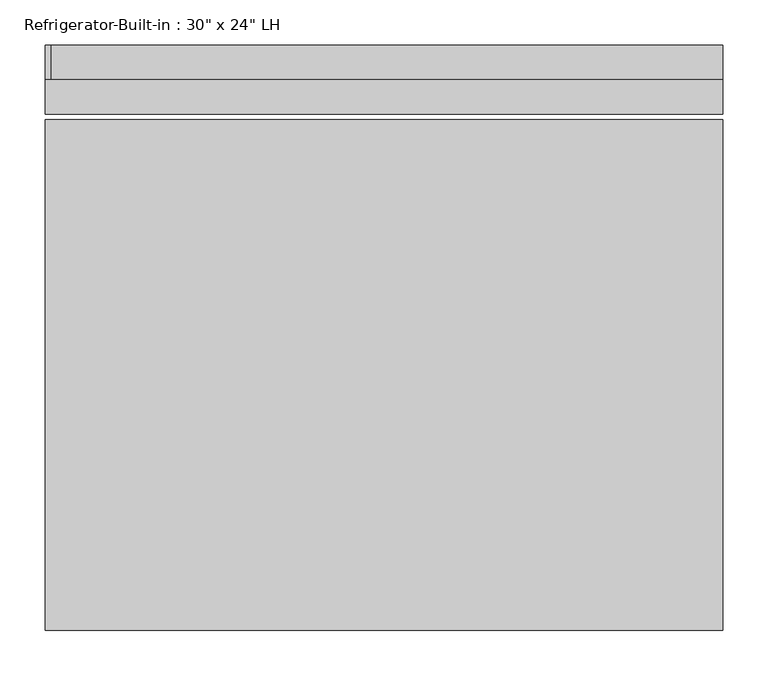
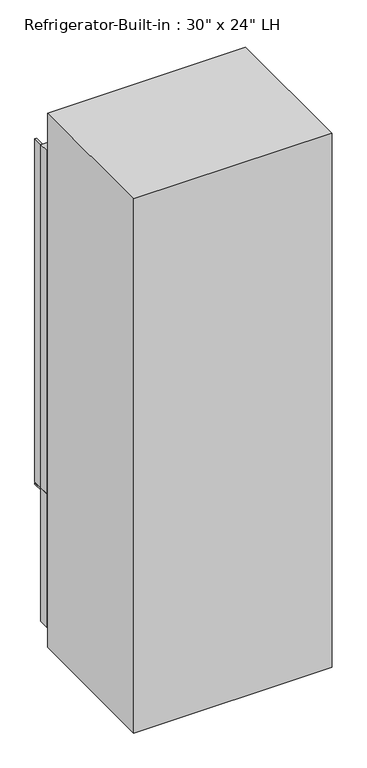
"""IFC4 building model written with IfcOpenShell, lengths in millimetres: proxy geometry."""

from ifc_helpers import new_model, si_unit, frame, origin, origin_with_axes, place, context, project, spatial, polyline, outline, extrude, source, transform, mapped, element, save


def proxy_76352e5b(model_context):
    return source(origin(), model_context, "Body", "SweptSolid", [
        extrude(outline(polyline([(374.65, -290.1239715), (-374.65, -290.1239715), (-374.65, 275.0260285), (374.65, 275.0260285), (374.65, -290.1239715)])), origin_with_axes(), (0.0, 0.0, 1.0), 2133.6),
        extrude(outline(polyline([(374.65, 281.3760285), (-374.65, 281.3760285), (-374.65, 319.4760285), (374.65, 319.4760285), (374.65, 281.3760285)])), frame((0.0, 0.0, 611.1875), z_axis=(0.0, 0.0, 1.0), x_axis=(1.0, 0.0, 0.0)), (0.0, 0.0, 1.0), 1370.0125),
        extrude(outline(polyline([(374.65, 281.3760285), (-374.65, 281.3760285), (-374.65, 319.4760285), (374.65, 319.4760285), (374.65, 281.3760285)])), frame((0.0, 0.0, 76.2), z_axis=(0.0, 0.0, 1.0), x_axis=(1.0, 0.0, 0.0)), (0.0, 0.0, 1.0), 531.8125),
        extrude(outline(polyline([(374.65, 319.4760285), (-374.65, 319.4760285), (-374.65, 357.5760285), (374.65, 357.5760285), (374.65, 319.4760285)])), frame((0.0, 0.0, 601.6625), z_axis=(0.0, 0.0, 1.0), x_axis=(1.0, 0.0, 0.0)), (0.0, 0.0, 1.0), 6.35),
        extrude(outline(polyline([(-374.65, 319.4760285), (-374.65, 357.5760285), (-368.3, 357.5760285), (-368.3, 319.4760285), (-374.65, 319.4760285)])), frame((0.0, 0.0, 611.1875), z_axis=(0.0, 0.0, 1.0), x_axis=(1.0, 0.0, 0.0)), (0.0, 0.0, 1.0), 1370.0125),
    ])


if __name__ == "__main__":
    model = new_model("IFC4")
    model_context = context("Model", 3, world=origin())
    ifc_project = project(units=[si_unit("LENGTHUNIT", "METRE", prefix="MILLI")], contexts=[model_context])
    site = spatial("IfcSite", under=ifc_project)
    building = spatial("IfcBuilding", under=site)
    placement = place(None, origin())
    proxy_shape = proxy_76352e5b(model_context)
    element("IfcBuildingElementProxy", 1, Name="Refrigerator-Built-in : 30\" x 24\" LH", ObjectType="Refrigerator-Built-in : 30\" x 24\" LH", at=placement, inside=building, context=model_context, shape_type="MappedRepresentation", body=[
        mapped(proxy_shape, transform((0.0, 0.0, 0.0), x_axis=(1.0, 0.0, 0.0), y_axis=(0.0, 1.0, 0.0), z_axis=(0.0, 0.0, 1.0))),
    ])
    save(model, "model.ifc")

# Revit data of these elements
# Type "Refrigerator-Built-in : 30\" x 24\" LH"
#   Assembly Code = "E1090400"
#   Depth = 2' - 0"
#   Handle = 0' - 0 1/4"
#   Height = 7' - 0"
#   Top Door Height = 5' - 0"
#   Width = 2' - 5 1/2"
#   Material = Metal - Paint Finish - Ivory,Glossy
#   Default Elevation = 0
# Element 1 (IfcBuildingElementProxy, "Refrigerator-Built-in : 30\" x 24\" LH")
#   Materials on its faces: "Metal - Paint Finish - Ivory,Glossy", "Metal - Chrome"
# Materials
#   "Metal - Paint Finish - Ivory,Glossy": colour RGB 247 247 239, transparency 0
#   "Metal - Chrome": colour RGB 57 57 57, transparency 0
